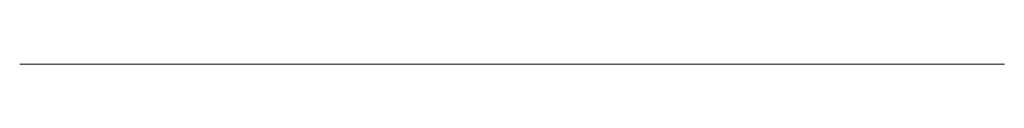
# Model space of a CAD drawing. Units: millimetres. Extents: x 248 to 348, y 0 to 0.
import ezdxf

# ---------------------------------------------------------------- set-up
doc = ezdxf.new("R2010")
doc.units = ezdxf.units.MM
doc.layers.add('M-CONS', color=8, linetype='Continuous', lineweight=18)

msp = doc.modelspace()

# ---------------------------------------------------------------- linework, layer by layer
at = {"layer": 'M-CONS', "extrusion": (0, -1, 0)}
msp.add_lwpolyline([(348.38, 149.1), (248.38, 149.1), (248.38, 139.1), (348.38, 139.1)], close=True, dxfattribs=at)

doc.saveas('drawing.dxf')
